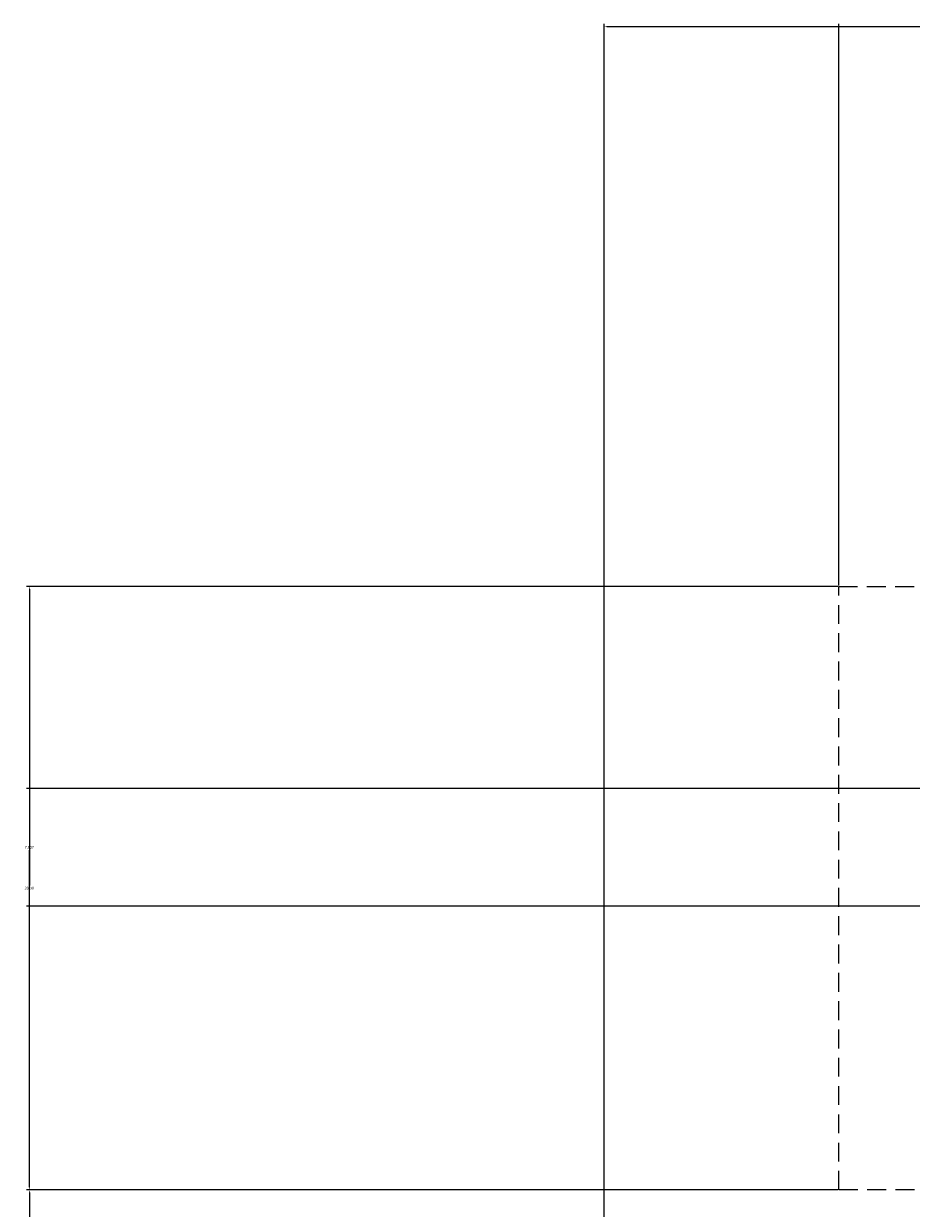
# Model space of a CAD drawing. Units: inches. Extents: x 412 to 584, y 208 to 437.
# Tile 16 of 28: x 412 to 471, y 359 to 437. Entities that reach past the tile are written whole.
import ezdxf

# ---------------------------------------------------------------- set-up
doc = ezdxf.new("R2010")
doc.units = ezdxf.units.IN
doc.header["$MEASUREMENT"] = 0
doc.linetypes.add('HIDDEN', pattern=[0.375, 0.25, -0.125])
doc.layers.add('A-ANNO-DIMS', color=2, linetype='Continuous', lineweight=18)
doc.layers.add('E-ENCL-HIDN', color=3, linetype='HIDDEN', lineweight=18)
doc.styles.get("Standard").update_dxf_attribs({"font": 'arial.ttf'})
doc.dimstyles.get("Standard").update_dxf_attribs({"dimtxt": 0.18, "dimasz": 0.18, "dimexe": 0.18, "dimexo": 0.0625, "dimgap": 0.09, "dimtad": 0, "dimtih": 1, "dimtoh": 1, "dimdec": 4, "dimzin": 0, "dimdsep": 46, "dimtxsty": 'Standard', "dimcen": 0.09, "dimadec": 0, "dimazin": 0, "dimtfac": 1, "dimtdec": 4, "dimtofl": 0, "dimtmove": 0, "dimatfit": 3, "dimfxl": 1, "dimtolj": 1, "dimtzin": 0, "dimarcsym": 0})

# ---------------------------------------------------------------- blocks, each defined once
blk = doc.blocks.new('*D21')
at = {"layer": 'A-ANNO-DIMS', "color": 0, "lineweight": -2, "transparency": 16777216}
for p, q in [((466.104, 400.237), (466.104, 437.465)), ((466.284, 437.285), (501.986, 437.285)), ((538.439, 437.285), (502.737, 437.285)), ((538.619, 400.237), (538.619, 437.465))]:
    blk.add_line(p, q, dxfattribs=at)
at = {"layer": 'A-ANNO-DIMS', "color": 0, "transparency": 16777216}
for points in [[(466.284, 437.315), (466.284, 437.255), (466.104, 437.285)], [(538.439, 437.315), (538.439, 437.255), (538.619, 437.285)]]:
    blk.add_solid(points, dxfattribs=at)
at = {"layer": 'Defpoints', "color": 0, "transparency": 16777216}
for p in [(538.619, 437.285), (466.104, 400.175), (538.619, 400.175)]:
    blk.add_point(p, dxfattribs=at)
at = {"layer": 'A-ANNO-DIMS', "color": 0, "transparency": 16777216, "insert": (502.361, 437.285), "char_height": 0.18, "attachment_point": 5}
blk.add_mtext('\\A1;72.51', dxfattribs=at)
blk = doc.blocks.new('*D22')
at = {"layer": 'A-ANNO-DIMS', "color": 0, "lineweight": -2, "transparency": 16777216}
for p, q in [((466.041, 400.175), (412.276, 400.175)), ((412.456, 399.995), (412.456, 380.367)), ((412.456, 360.376), (412.456, 380.004)), ((466.041, 360.196), (412.276, 360.196))]:
    blk.add_line(p, q, dxfattribs=at)
at = {"layer": 'A-ANNO-DIMS', "color": 0, "transparency": 16777216}
for points in [[(412.426, 399.995), (412.486, 399.995), (412.456, 400.175)], [(412.426, 360.376), (412.486, 360.376), (412.456, 360.196)]]:
    blk.add_solid(points, dxfattribs=at)
at = {"layer": 'Defpoints', "color": 0, "transparency": 16777216}
for p in [(466.104, 400.175), (412.456, 360.196), (466.104, 360.196)]:
    blk.add_point(p, dxfattribs=at)
at = {"layer": 'A-ANNO-DIMS', "color": 0, "transparency": 16777216, "insert": (412.456, 380.186), "char_height": 0.18, "attachment_point": 5}
blk.add_mtext('\\A1;39.98', dxfattribs=at)
blk = doc.blocks.new('*D23')
at = {"layer": 'A-ANNO-DIMS', "color": 0, "lineweight": -2, "transparency": 16777216}
for p, q in [((466.041, 360.196), (412.276, 360.196)), ((412.456, 360.016), (412.456, 354.967)), ((412.456, 349.553), (412.456, 354.603)), ((499.225, 349.373), (412.276, 349.373))]:
    blk.add_line(p, q, dxfattribs=at)
at = {"layer": 'A-ANNO-DIMS', "color": 0, "transparency": 16777216}
for points in [[(412.426, 360.016), (412.486, 360.016), (412.456, 360.196)], [(412.426, 349.553), (412.486, 349.553), (412.456, 349.373)]]:
    blk.add_solid(points, dxfattribs=at)
at = {"layer": 'Defpoints', "color": 0, "transparency": 16777216}
for p in [(466.104, 360.196), (412.456, 349.373), (499.288, 349.373)]:
    blk.add_point(p, dxfattribs=at)
at = {"layer": 'A-ANNO-DIMS', "color": 0, "transparency": 16777216, "insert": (412.456, 354.785), "char_height": 0.18, "attachment_point": 5}
blk.add_mtext('\\A1;10.823', dxfattribs=at)
blk = doc.blocks.new('*D27')
at = {"layer": 'A-ANNO-DIMS', "color": 0, "lineweight": -2, "transparency": 16777216}
for p, q in [((466.104, 400.237), (466.104, 437.465)), ((466.284, 437.285), (482.233, 437.285)), ((499.108, 437.285), (483.159, 437.285)), ((499.288, 397.825), (499.288, 437.465))]:
    blk.add_line(p, q, dxfattribs=at)
at = {"layer": 'A-ANNO-DIMS', "color": 0, "transparency": 16777216}
for points in [[(466.284, 437.315), (466.284, 437.255), (466.104, 437.285)], [(499.108, 437.315), (499.108, 437.255), (499.288, 437.285)]]:
    blk.add_solid(points, dxfattribs=at)
at = {"layer": 'Defpoints', "color": 0, "transparency": 16777216}
for p in [(499.288, 437.285), (466.104, 400.175), (499.288, 397.763)]:
    blk.add_point(p, dxfattribs=at)
at = {"layer": 'A-ANNO-DIMS', "color": 0, "transparency": 16777216, "insert": (482.696, 437.285), "char_height": 0.18, "attachment_point": 5}
blk.add_mtext('\\A1;33.184', dxfattribs=at)
blk = doc.blocks.new('*D28')
at = {"layer": 'A-ANNO-DIMS', "color": 0, "lineweight": -2, "transparency": 16777216}
for p, q in [((450.562, 256.635), (450.562, 437.465)), ((450.742, 437.285), (502.724, 437.285)), ((555.616, 437.285), (503.634, 437.285)), ((555.796, 256.635), (555.796, 437.465))]:
    blk.add_line(p, q, dxfattribs=at)
at = {"layer": 'A-ANNO-DIMS', "color": 0, "transparency": 16777216}
for points in [[(450.742, 437.315), (450.742, 437.255), (450.562, 437.285)], [(555.616, 437.315), (555.616, 437.255), (555.796, 437.285)]]:
    blk.add_solid(points, dxfattribs=at)
at = {"layer": 'Defpoints', "color": 0, "transparency": 16777216}
for p in [(555.796, 437.285), (450.562, 256.573), (555.796, 256.573)]:
    blk.add_point(p, dxfattribs=at)
at = {"layer": 'A-ANNO-DIMS', "color": 0, "transparency": 16777216, "insert": (503.179, 437.285), "char_height": 0.18, "attachment_point": 5}
blk.add_mtext('\\A1;105.23', dxfattribs=at)
blk = doc.blocks.new('*D30')
at = {"layer": 'A-ANNO-DIMS', "color": 0, "lineweight": -2, "transparency": 16777216}
for p, q in [((495.864, 386.793), (412.276, 386.793)), ((412.456, 386.613), (412.456, 383.072)), ((412.456, 379.167), (412.456, 382.708)), ((495.864, 378.987), (412.276, 378.987))]:
    blk.add_line(p, q, dxfattribs=at)
at = {"layer": 'A-ANNO-DIMS', "color": 0, "transparency": 16777216}
for points in [[(412.426, 386.613), (412.486, 386.613), (412.456, 386.793)], [(412.426, 379.167), (412.486, 379.167), (412.456, 378.987)]]:
    blk.add_solid(points, dxfattribs=at)
at = {"layer": 'Defpoints', "color": 0, "transparency": 16777216}
for p in [(495.927, 386.793), (412.456, 378.987), (495.927, 378.987)]:
    blk.add_point(p, dxfattribs=at)
at = {"layer": 'A-ANNO-DIMS', "color": 0, "transparency": 16777216, "insert": (412.456, 382.89), "char_height": 0.18, "attachment_point": 5}
blk.add_mtext('\\A1;7.807', dxfattribs=at)

msp = doc.modelspace()

# ---------------------------------------------------------------- linework, layer by layer
at = {"layer": 'E-ENCL-HIDN', "ltscale": 5}
msp.add_lwpolyline([(466.1037, 400.175), (538.6186, 400.175), (538.6186, 360.1961), (466.1037, 360.1961)], close=True, dxfattribs=at)

# ---------------------------------------------------------------- dimensions: what is measured, and where the dimension line sits
at = {"layer": 'A-ANNO-DIMS'}
for base, p1, p2, override, picture, middle in [((555.7959, 437.2847), (450.562, 256.5729), (555.7959, 256.5729), {"dimdec": 2, "dimlfac": 1, "dimrnd": 0, "dimzin": 0, "dimdsep": 46, "dimlunit": 2}, '*D28', (503.1789, 437.2847)), ((538.6186, 437.2847), (466.1037, 400.175), (538.6186, 400.175), {"dimdec": 2, "dimlfac": 1, "dimrnd": 0, "dimzin": 0, "dimdsep": 46, "dimlunit": 2}, '*D21', (502.3612, 437.2847)), ((499.2878, 437.2847), (466.1037, 400.175), (499.2878, 397.7626), {"dimdec": 3, "dimlfac": 1, "dimrnd": 0, "dimzin": 0, "dimdsep": 46, "dimlunit": 2}, '*D27', (482.6958, 437.2847))]:
    dim = msp.add_linear_dim(base=base, p1=p1, p2=p2, dimstyle='Standard', override=override, dxfattribs=at)
    dim.commit()
    dim.dimension.update_dxf_attribs({"geometry": picture, "text_midpoint": middle})
for base, p1, p2, override, picture, middle in [((412.4562, 360.1961), (466.1037, 400.175), (466.1037, 360.1961), {"dimdec": 2, "dimlfac": 1, "dimrnd": 0, "dimzin": 0, "dimdsep": 46, "dimlunit": 2}, '*D22', (412.4562, 380.1855)), ((412.4562, 378.9867), (495.9268, 386.7933), (495.9268, 378.9867), {"dimdec": 3, "dimlfac": 1, "dimrnd": 0, "dimzin": 0, "dimdsep": 46, "dimlunit": 2}, '*D30', (412.4562, 382.89)), ((412.4562, 349.3734), (466.1037, 360.1961), (499.2878, 349.3734), {"dimdec": 3, "dimlfac": 1, "dimrnd": 0, "dimzin": 0, "dimdsep": 46, "dimlunit": 2}, '*D23', (412.4562, 354.7847))]:
    dim = msp.add_linear_dim(base=base, p1=p1, p2=p2, angle=90, dimstyle='Standard', override=override, dxfattribs=at)
    dim.commit()
    dim.dimension.update_dxf_attribs({"geometry": picture, "text_midpoint": middle})

doc.saveas('drawing.dxf')
